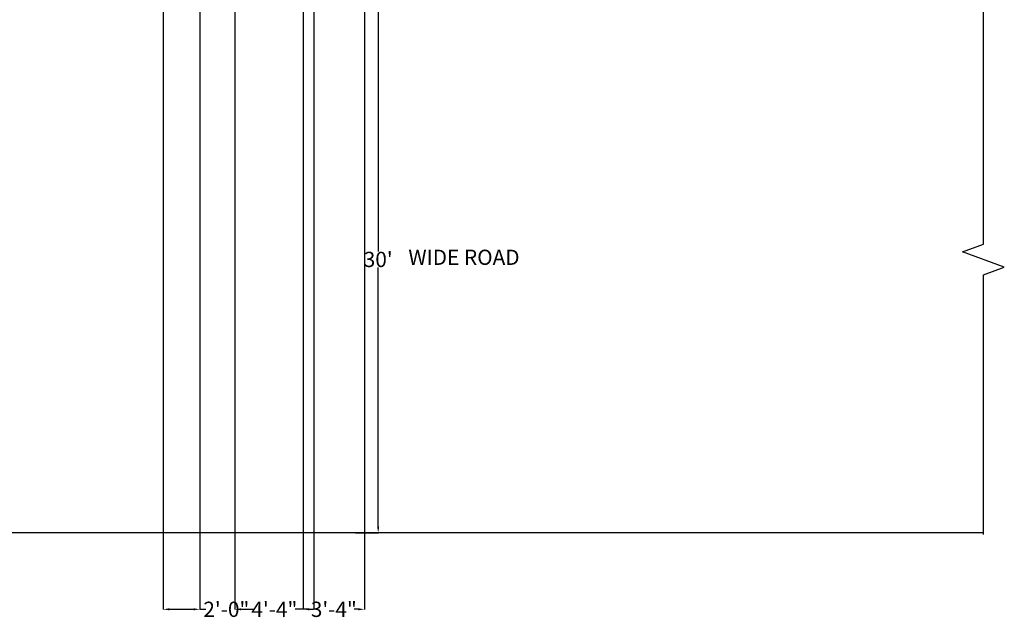
# Model space of a CAD drawing. Units: inches. Extents: x 529 to 1659, y 271 to 1222.
# Tile 2 of 5: x 936 to 1581, y 271 to 664. Entities that reach past the tile are written whole.
import ezdxf

# ---------------------------------------------------------------- set-up
doc = ezdxf.new("R2010")
doc.units = ezdxf.units.IN
doc.header["$MEASUREMENT"] = 0
for name, color, linetype, lineweight in [('C-ROAD', 7, 'Continuous', 25), ('DIM', 241, 'Continuous', 18), ('TEXT', 131, 'Continuous', 18)]:
    doc.layers.add(name, color=color, linetype=linetype, lineweight=lineweight)
doc.styles.get("Standard").update_dxf_attribs({"font": 'arial.ttf', "height": 10})
doc.dimstyles.get("Standard").update_dxf_attribs({"dimtxt": 6, "dimasz": 4, "dimexe": 0.18, "dimexo": 0.0625, "dimgap": 0.09, "dimtad": 0, "dimtih": 1, "dimtoh": 1, "dimdec": 0, "dimrnd": 6, "dimzin": 0, "dimdsep": 46, "dimlunit": 3, "dimtxsty": 'Standard', "dimcen": 0.09, "dimadec": 0, "dimazin": 0, "dimtfac": 1, "dimtdec": 0, "dimtofl": 0, "dimtmove": 0, "dimatfit": 3, "dimfxl": 1, "dimtolj": 1, "dimtzin": 0, "dimarcsym": 0})

# ---------------------------------------------------------------- blocks, each defined once
blk = doc.blocks.new('*D8')
at = {"layer": 'Defpoints', "color": 0, "transparency": 16777216}
for p in [(1155.49, 685.86), (1170.49, 685.86), (1155.55, 327.24)]:
    blk.add_point(p, dxfattribs=at)
at = {"layer": 'DIM', "color": 0, "lineweight": -2, "transparency": 16777216}
for p, q in [((1155.56, 685.86), (1170.67, 685.86)), ((1170.49, 681.86), (1170.49, 511.75)), ((1170.49, 331.24), (1170.49, 501.35)), ((1155.61, 327.24), (1170.67, 327.24))]:
    blk.add_line(p, q, dxfattribs=at)
at = {"layer": 'DIM', "color": 0, "transparency": 16777216}
for points in [[(1169.83, 681.86), (1171.16, 681.86), (1170.49, 685.86)], [(1169.83, 331.24), (1171.16, 331.24), (1170.49, 327.24)]]:
    blk.add_solid(points, dxfattribs=at)
at = {"layer": 'DIM', "color": 0, "transparency": 16777216, "insert": (1170.49, 506.55), "char_height": 10, "attachment_point": 5}
blk.add_mtext("\\A1;30'", dxfattribs=at)
blk = doc.blocks.new('ROAD-BREAKLINE')
blk.add_lwpolyline([(13.74, 0), (13.74, 170.31), (27.47, 175.31), (0, 185.31), (13.74, 190.31), (13.74, 360.62)])
blk = doc.blocks.new('*D29')
at = {"layer": 'Defpoints', "color": 0, "transparency": 16777216}
for p in [(1076.49, 941.86), (1128.41, 941.86), (1128.41, 277.14)]:
    blk.add_point(p, dxfattribs=at)
at = {"layer": 'DIM', "color": 0, "lineweight": -2, "transparency": 16777216}
for p, q in [((1076.49, 941.79), (1076.49, 276.96)), ((1128.41, 941.79), (1128.41, 276.96)), ((1080.49, 277.14), (1088.87, 277.14)), ((1124.41, 277.14), (1116.04, 277.14))]:
    blk.add_line(p, q, dxfattribs=at)
at = {"layer": 'DIM', "color": 0, "transparency": 16777216}
for points in [[(1080.49, 277.81), (1080.49, 276.47), (1076.49, 277.14)], [(1124.41, 277.81), (1124.41, 276.47), (1128.41, 277.14)]]:
    blk.add_solid(points, dxfattribs=at)
at = {"layer": 'DIM', "color": 0, "transparency": 16777216, "insert": (1102.45, 277.14), "char_height": 10, "attachment_point": 5}
blk.add_mtext('\\A1;4\'-4"', dxfattribs=at)
blk = doc.blocks.new('*D31')
at = {"layer": 'Defpoints', "color": 0, "transparency": 16777216}
for p in [(1121.32, 736.86), (1161.49, 736.86), (1161.49, 277.14)]:
    blk.add_point(p, dxfattribs=at)
at = {"layer": 'DIM', "color": 0, "lineweight": -2, "transparency": 16777216}
for p, q in [((1121.32, 736.79), (1121.32, 276.96)), ((1161.49, 736.79), (1161.49, 276.96)), ((1125.32, 277.14), (1128.03, 277.14)), ((1157.49, 277.14), (1154.78, 277.14))]:
    blk.add_line(p, q, dxfattribs=at)
at = {"layer": 'DIM', "color": 0, "transparency": 16777216}
for points in [[(1125.32, 277.81), (1125.32, 276.47), (1121.32, 277.14)], [(1157.49, 277.81), (1157.49, 276.47), (1161.49, 277.14)]]:
    blk.add_solid(points, dxfattribs=at)
at = {"layer": 'DIM', "color": 0, "transparency": 16777216, "insert": (1141.41, 277.14), "char_height": 10, "attachment_point": 5}
blk.add_mtext('\\A1;3\'-4"', dxfattribs=at)
blk = doc.blocks.new('*D36')
at = {"layer": 'Defpoints', "color": 0, "transparency": 16777216}
for p in [(1029.49, 1126.86), (1053.49, 1102.86), (1053.49, 277.14)]:
    blk.add_point(p, dxfattribs=at)
at = {"layer": 'DIM', "color": 0, "lineweight": -2, "transparency": 16777216}
for p, q in [((1029.49, 1126.79), (1029.49, 276.96)), ((1053.49, 1102.79), (1053.49, 276.96)), ((1033.49, 277.14), (1049.49, 277.14)), ((1053.49, 277.14), (1057.49, 277.14))]:
    blk.add_line(p, q, dxfattribs=at)
at = {"layer": 'DIM', "color": 0, "transparency": 16777216}
for points in [[(1033.49, 277.81), (1033.49, 276.47), (1029.49, 277.14)], [(1049.49, 277.81), (1049.49, 276.47), (1053.49, 277.14)]]:
    blk.add_solid(points, dxfattribs=at)
at = {"layer": 'DIM', "color": 0, "transparency": 16777216, "insert": (1070.96, 277.14), "char_height": 10, "attachment_point": 5}
blk.add_mtext('\\A1;2\'-0"', dxfattribs=at)

msp = doc.modelspace()

# ---------------------------------------------------------------- linework, layer by layer
at = {"layer": 'C-ROAD'}
msp.add_line((1567.16, 327.24), (618.33, 327.24), dxfattribs=at)

# ---------------------------------------------------------------- block references
msp.add_blockref('ROAD-BREAKLINE', (1553.43, 326.24), dxfattribs=at)

# ---------------------------------------------------------------- texts
at = {"layer": 'TEXT', "insert": (1114.56, 512.95), "char_height": 10, "attachment_point": 1}
msp.add_mtext_dynamic_manual_height_columns('\\pxqc;WIDE ROAD', width=224.347, gutter_width=50, heights=[0], dxfattribs=at)

# ---------------------------------------------------------------- dimensions: what is measured, and where the dimension line sits
at = {"layer": 'DIM'}
for base, p1, p2, picture, middle in [((1053.49, 277.14), (1029.49, 1126.86), (1053.49, 1102.86), '*D36', (1070.96, 277.14)), ((1128.41, 277.14), (1076.49, 941.86), (1128.41, 941.86), '*D29', (1102.45, 277.14)), ((1161.49, 277.14), (1121.32, 736.86), (1161.49, 736.86), '*D31', (1141.41, 277.14))]:
    dim = msp.add_linear_dim(base=base, p1=p1, p2=p2, dimstyle='Standard', override={"dimdec": 1, "dimlfac": 1, "dimrnd": 0, "dimzin": 1, "dimdsep": 46, "dimlunit": 4, "dimfrac": 2}, dxfattribs=at)
    dim.commit()
    dim.dimension.update_dxf_attribs({"geometry": picture, "text_midpoint": middle})
dim = msp.add_linear_dim(base=(1170.49, 685.86), p1=(1155.55, 327.24), p2=(1155.49, 685.86), angle=90, dimstyle='Standard', override={"dimclrd": 0, "dimclre": 0, "dimclrt": 0}, dxfattribs=at)
dim.commit()
dim.dimension.update_dxf_attribs({"geometry": '*D8', "text_midpoint": (1170.49, 506.55)})

doc.saveas('drawing.dxf')
